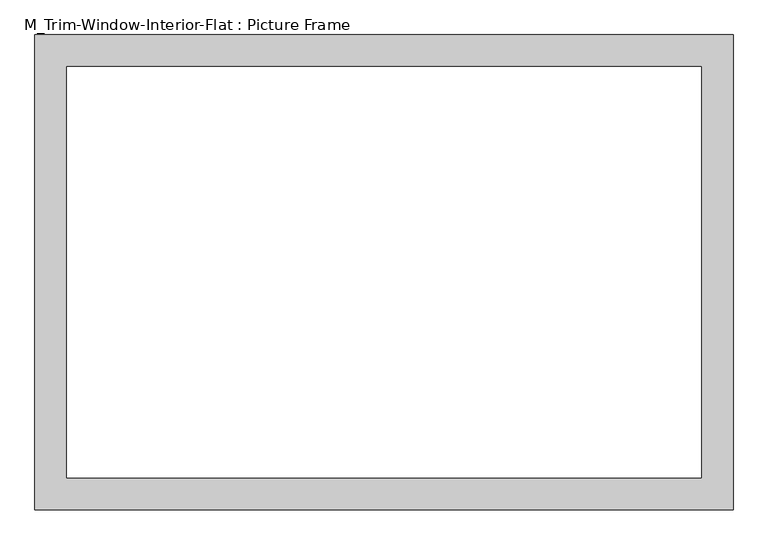
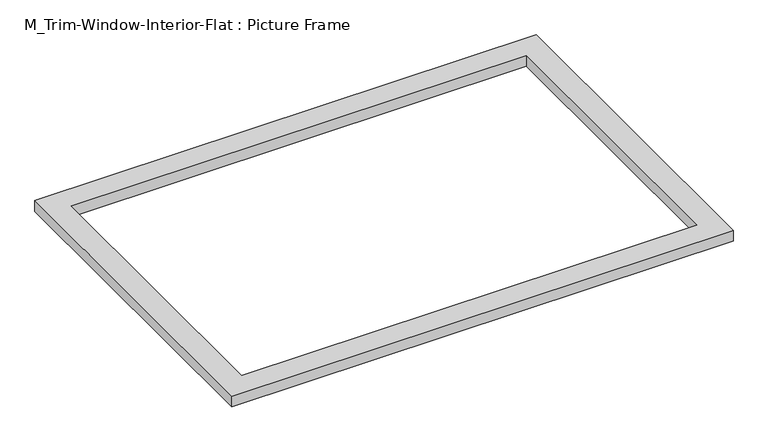
"""IFC4 building model written with IfcOpenShell, lengths in millimetres: proxy geometry, M_Trim-Window-Interior-Flat : Picture Frame."""

from ifc_helpers import new_model, si_unit, origin, origin_with_axes, place, context, project, spatial, polyline, outline, extrude, source, transform, mapped, element, save


def m_trim_window_interior_flat_picture_frame_7ff13b15(model_context):
    return source(origin(), model_context, "Body", "SweptSolid", [
        extrude(outline(polyline([(656.9, -47.3), (-656.9, -47.3), (-656.9, 847.3), (656.9, 847.3), (656.9, -47.3)]), holes=[polyline([(596.9, 12.7), (596.9, 787.3), (-596.9, 787.3), (-596.9, 12.7), (596.9, 12.7)])]), origin_with_axes(), (0.0, 0.0, 1.0), 30.0),
    ])


if __name__ == "__main__":
    model = new_model("IFC4")
    model_context = context("Model", 3, world=origin())
    ifc_project = project(units=[si_unit("LENGTHUNIT", "METRE", prefix="MILLI")], contexts=[model_context])
    site = spatial("IfcSite", under=ifc_project)
    building = spatial("IfcBuilding", under=site)
    placement = place(None, origin())
    m_trim_window_interior_flat_picture_frame_shape = m_trim_window_interior_flat_picture_frame_7ff13b15(model_context)
    element("IfcBuildingElementProxy", 1, Name="M_Trim-Window-Interior-Flat : Picture Frame", ObjectType="M_Trim-Window-Interior-Flat : Picture Frame", at=placement, inside=building, context=model_context, shape_type="MappedRepresentation", body=[
        mapped(m_trim_window_interior_flat_picture_frame_shape, transform((0.0, 0.0, 0.0), x_axis=(1.0, 0.0, 0.0), y_axis=(0.0, 1.0, 0.0), z_axis=(0.0, 0.0, 1.0))),
    ])
    save(model, "model.ifc")

# Revit data of these elements
# Type "M_Trim-Window-Interior-Flat : Picture Frame"
#   Trim Thickness_Picture Frame = 0' - 1.1811"
#   Trim Width = 0' - 2.3622"
#   Trim Thickness_with Sill = 0' - 0.7874"
#   Sill Thickness = 0' - 1.1811"
#   Opening Width [instance default] = 1' - 11.62205"
#   Opening Height [instance default] = 2' - 11.43307"
#   Default Elevation = 3' - 11.24409"
#   Sill = no
#   Picture Frame = yes
#   Trim Material [instance default] = none
# Element 1 (IfcBuildingElementProxy, "M_Trim-Window-Interior-Flat : Picture Frame")
#   Opening Width = 4' - 0"
#   Opening Height = 2' - 7.49606"
#   Trim Material = Wood - Stained
#   Materials on its faces: "Wood - Stained"
# Materials
#   "Wood - Stained": class "Wood", colour RGB 224 178 126, transparency 0, Cost = 0
